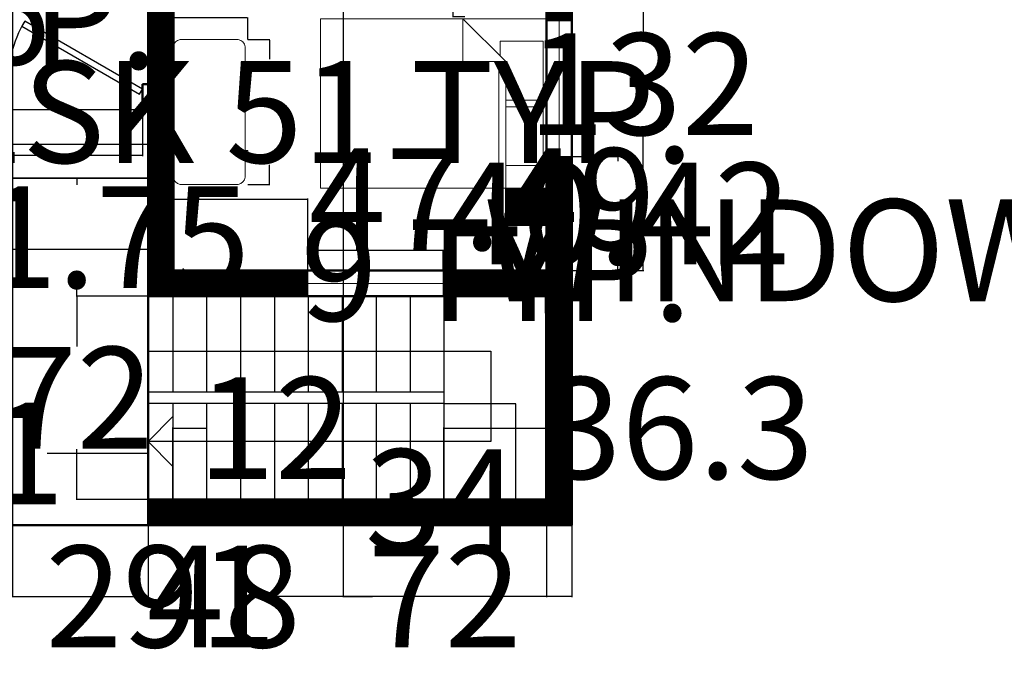
# Model space of a CAD drawing. Units: inches. Extents: x 1173 to 2157, y 515 to 1129.
# Tile 4 of 13: x 1475 to 1824, y 515 to 743. Entities that reach past the tile are written whole.
import ezdxf

# ---------------------------------------------------------------- set-up
doc = ezdxf.new("R2010")
doc.units = ezdxf.units.IN
doc.header["$MEASUREMENT"] = 0
for name, color, linetype, lineweight in [('A-ANNO-DIMS', 2, 'Continuous', 18), ('A-DOOR', 3, 'Continuous', 25), ('A-FLOR', 7, 'Continuous', 25), ('A-FLOR-STRS', 7, 'Continuous', 25), ('A-FURN', 8, 'Continuous', 18), ('A-GLAZ', 4, 'Continuous', 18), ('A-WALL', 7, 'Continuous', 50)]:
    doc.layers.add(name, color=color, linetype=linetype, lineweight=lineweight)
doc.layers.add('A-FURN-PATT', color=7, linetype='Continuous', lineweight=13, true_color=0xffffff)
doc.layers.add('A-WALL-PATT', color=22, linetype='Continuous', lineweight=13, true_color=0xca4b0c)
doc.styles.get("Standard").update_dxf_attribs({"font": 'arial.ttf'})
doc.dimstyles.get("Standard").update_dxf_attribs({"dimtxt": 36, "dimasz": 0.18, "dimexe": 0.18, "dimexo": 0.0625, "dimgap": 0.09, "dimtad": 0, "dimtih": 1, "dimtoh": 1, "dimdec": 0, "dimrnd": 72, "dimzin": 0, "dimdsep": 46, "dimlunit": 3, "dimtxsty": 'Standard', "dimcen": 2, "dimadec": 0, "dimazin": 0, "dimtfac": 1, "dimtdec": 0, "dimtofl": 0, "dimtmove": 0, "dimatfit": 3, "dimfxl": 1, "dimtolj": 1, "dimtzin": 0, "dimarcsym": 0})

# ---------------------------------------------------------------- blocks, each defined once
blk = doc.blocks.new('*U2')
for p, q in [((0, 0), (0, -6)), ((-40, 0), (-40, -6))]:
    blk.add_line(p, q)
blk.add_lwpolyline([(0, 0), (-34.64, 20), (-35.52, 18.48), (-0.88, -1.52)], close=True)
blk.add_arc((0, 0), 40, 150, 180)
blk = doc.blocks.new('Bed - Queen')
for p, q in [((0, -80.00003), (0, 0)), ((0, 0), (59.99999, 0)), ((59.99999, 0), (59.99999, -80.00003)), ((7.99999, -1.2), (28.79998, -1.2)), ((7.99999, -14.4), (7.99999, -1.2)), ((28.79998, -1.2), (28.79998, -14.4)), ((31.19999, -1.2), (51.99999, -1.2)), ((31.19999, -14.4), (31.19999, -1.2)), ((51.99999, -1.2), (51.99999, -16.4)), ((0, -14.4), (44.8, -14.4)), ((44.8, -16.8), (0, -16.8)), ((59.99999, -29.6), (44.8, -14.4)), ((44.8, -14.4), (44.8, -29.6)), ((51.99999, -16.4), (46.79936, -16.4)), ((44.8, -29.6), (59.99999, -29.6)), ((59.99999, -80.00003), (0, -80.00003))]:
    blk.add_line(p, q)
blk = doc.blocks.new('Desk - 30 x 60 in.')
for p, q in [((-26.999995, 0), (26.999995, 0)), ((-29.999995, -27), (-29.999995, -3)), ((29.999995, -3), (29.999995, -27)), ((26.999995, -30), (-26.999995, -30)), ((-20.000005, -30), (-20.000005, -31)), ((-20.000005, -31), (-16.000005, -31)), ((-16.000005, -31), (-16.000005, -30)), ((15.999995, -31), (15.999995, -30)), ((19.999995, -31), (15.999995, -31)), ((19.999995, -30), (19.999995, -31))]:
    blk.add_line(p, q)
for centre, start, end in [((-26.499995, -3.5), 98.1301, 171.8699), ((26.499995, -3.5), 8.130102, 81.8699), ((-26.499995, -26.5), 188.1301, 261.8699), ((26.499995, -26.5), 278.1301, 351.8699)]:
    blk.add_arc(centre, 3.535534, start, end)
blk = doc.blocks.new('WIN-48X9')
blk.add_line((48, 4.5), (0, 4.5))
blk.add_lwpolyline([(0, 9), (48, 9), (48, 0), (0, 0)], close=True)
blk = doc.blocks.new('*D26')
at = {"layer": 'A-ANNO-DIMS', "color": 0, "lineweight": -2, "transparency": 16777216}
for p, q in [((1577.15, 654.34), (1577.15, 661.66)), ((1577.33, 661.48), (1624.97, 661.48)), ((1625.15, 654.34), (1625.15, 661.66)), ((1625.15, 661.48), (1625.33, 661.48))]:
    blk.add_line(p, q, dxfattribs=at)
at = {"layer": 'A-ANNO-DIMS', "color": 0, "transparency": 16777216}
for points in [[(1577.33, 661.51), (1577.33, 661.45), (1577.15, 661.48)], [(1624.97, 661.51), (1624.97, 661.45), (1625.15, 661.48)]]:
    blk.add_solid(points, dxfattribs=at)
at = {"layer": 'Defpoints', "color": 0, "transparency": 16777216}
for p in [(1625.15, 661.48), (1577.15, 654.28), (1625.15, 654.28)]:
    blk.add_point(p, dxfattribs=at)
at = {"layer": 'A-ANNO-DIMS', "color": 0, "transparency": 16777216, "insert": (1831.09, 661.48), "char_height": 36, "attachment_point": 5}
blk.add_mtext('\\A1;WINDOW 48 TYP.', dxfattribs=at)
blk = doc.blocks.new('*D27')
at = {"layer": 'A-ANNO-DIMS', "color": 0, "lineweight": -2, "transparency": 16777216}
for p, q in [((1577.09, 654.28), (1569.77, 654.28)), ((1569.95, 654.28), (1569.95, 654.46)), ((1569.95, 654.46), (1570.13, 654.46)), ((1569.95, 645.46), (1569.95, 654.1)), ((1577.09, 645.28), (1569.77, 645.28))]:
    blk.add_line(p, q, dxfattribs=at)
at = {"layer": 'A-ANNO-DIMS', "color": 0, "transparency": 16777216}
for points in [[(1569.92, 654.1), (1569.98, 654.1), (1569.95, 654.28)], [(1569.92, 645.46), (1569.98, 645.46), (1569.95, 645.28)]]:
    blk.add_solid(points, dxfattribs=at)
at = {"layer": 'Defpoints', "color": 0, "transparency": 16777216}
for p in [(1569.95, 654.28), (1577.15, 654.28), (1577.15, 645.28)]:
    blk.add_point(p, dxfattribs=at)
at = {"layer": 'A-ANNO-DIMS', "color": 0, "transparency": 16777216, "insert": (1643.85, 654.46), "char_height": 36, "attachment_point": 5}
blk.add_mtext('\\A1;9 TYP.', dxfattribs=at)
blk = doc.blocks.new('*D30')
at = {"layer": 'A-ANNO-DIMS', "color": 0, "lineweight": -2, "transparency": 16777216}
for p, q in [((1555.97, 736.03), (1563.78, 736.03)), ((1563.6, 735.85), (1563.6, 729.12)), ((1563.6, 684.97), (1563.6, 691.71)), ((1555.97, 684.79), (1563.78, 684.79))]:
    blk.add_line(p, q, dxfattribs=at)
at = {"layer": 'A-ANNO-DIMS', "color": 0, "transparency": 16777216}
for points in [[(1563.57, 735.85), (1563.63, 735.85), (1563.6, 736.03)], [(1563.57, 684.97), (1563.63, 684.97), (1563.6, 684.79)]]:
    blk.add_solid(points, dxfattribs=at)
at = {"layer": 'Defpoints', "color": 0, "transparency": 16777216}
for p in [(1555.91, 736.03), (1563.6, 736.03), (1555.91, 684.79)]:
    blk.add_point(p, dxfattribs=at)
at = {"layer": 'A-ANNO-DIMS', "color": 0, "transparency": 16777216, "insert": (1563.6, 710.41), "char_height": 36, "attachment_point": 5}
blk.add_mtext('\\A1;DESK 51 TYP.', dxfattribs=at)
blk = doc.blocks.new('*D31')
at = {"layer": 'A-ANNO-DIMS', "color": 0, "lineweight": -2, "transparency": 16777216}
for p, q in [((1529.44, 743.72), (1529.26, 743.72)), ((1529.44, 736.09), (1529.44, 743.9)), ((1555.73, 743.72), (1529.62, 743.72)), ((1555.91, 736.09), (1555.91, 743.9))]:
    blk.add_line(p, q, dxfattribs=at)
at = {"layer": 'A-ANNO-DIMS', "color": 0, "transparency": 16777216}
for points in [[(1529.62, 743.75), (1529.62, 743.69), (1529.44, 743.72)], [(1555.73, 743.75), (1555.73, 743.69), (1555.91, 743.72)]]:
    blk.add_solid(points, dxfattribs=at)
at = {"layer": 'Defpoints', "color": 0, "transparency": 16777216}
for p in [(1529.44, 743.72), (1529.44, 736.03), (1555.91, 736.03)]:
    blk.add_point(p, dxfattribs=at)
at = {"layer": 'A-ANNO-DIMS', "color": 0, "transparency": 16777216, "insert": (1441.24, 743.72), "char_height": 36, "attachment_point": 5}
blk.add_mtext('\\A1;26 TYP.', dxfattribs=at)
blk = doc.blocks.new('*D32')
at = {"layer": 'A-ANNO-DIMS', "color": 0, "lineweight": -2, "transparency": 16777216}
for p, q in [((1632.82, 772.28), (1632.82, 776.62)), ((1633, 776.44), (1660.73, 776.44)), ((1660.91, 772.28), (1660.91, 776.62)), ((1660.91, 776.44), (1661.09, 776.44))]:
    blk.add_line(p, q, dxfattribs=at)
at = {"layer": 'A-ANNO-DIMS', "color": 0, "transparency": 16777216}
for points in [[(1633, 776.47), (1633, 776.41), (1632.82, 776.44)], [(1660.73, 776.47), (1660.73, 776.41), (1660.91, 776.44)]]:
    blk.add_solid(points, dxfattribs=at)
at = {"layer": 'Defpoints', "color": 0, "transparency": 16777216}
for p in [(1660.91, 776.44), (1632.82, 772.22), (1660.91, 772.22)]:
    blk.add_point(p, dxfattribs=at)
at = {"layer": 'A-ANNO-DIMS', "color": 0, "transparency": 16777216, "insert": (1823.46, 776.44), "char_height": 36, "attachment_point": 5}
blk.add_mtext('\\A1;LAMP 28 TYP.', dxfattribs=at)
blk = doc.blocks.new('*D33')
at = {"layer": 'A-ANNO-DIMS', "color": 0, "lineweight": -2, "transparency": 16777216}
for p, q in [((1632.75, 772.22), (1628.42, 772.22)), ((1628.6, 772.22), (1628.6, 772.4)), ((1628.6, 772.4), (1628.78, 772.4)), ((1628.6, 744.31), (1628.6, 772.04)), ((1632.75, 744.13), (1628.42, 744.13))]:
    blk.add_line(p, q, dxfattribs=at)
at = {"layer": 'A-ANNO-DIMS', "color": 0, "transparency": 16777216}
for points in [[(1628.57, 772.04), (1628.63, 772.04), (1628.6, 772.22)], [(1628.57, 744.31), (1628.63, 744.31), (1628.6, 744.13)]]:
    blk.add_solid(points, dxfattribs=at)
at = {"layer": 'Defpoints', "color": 0, "transparency": 16777216}
for p in [(1628.6, 772.22), (1632.82, 772.22), (1632.82, 744.13)]:
    blk.add_point(p, dxfattribs=at)
at = {"layer": 'A-ANNO-DIMS', "color": 0, "transparency": 16777216, "insert": (1716.8, 772.4), "char_height": 36, "attachment_point": 5}
blk.add_mtext('\\A1;28 TYP.', dxfattribs=at)
blk = doc.blocks.new('*D50')
at = {"layer": 'A-ANNO-DIMS', "color": 0, "lineweight": -2, "transparency": 16777216}
for p, q in [((1603.33, 796.77), (1603.15, 796.77)), ((1603.33, 798.21), (1603.33, 796.59)), ((1613.15, 796.77), (1603.51, 796.77)), ((1613.33, 798.21), (1613.33, 796.59))]:
    blk.add_line(p, q, dxfattribs=at)
at = {"layer": 'A-ANNO-DIMS', "color": 0, "transparency": 16777216}
for points in [[(1603.51, 796.8), (1603.51, 796.74), (1603.33, 796.77)], [(1613.15, 796.8), (1613.15, 796.74), (1613.33, 796.77)]]:
    blk.add_solid(points, dxfattribs=at)
at = {"layer": 'Defpoints', "color": 0, "transparency": 16777216}
for p in [(1603.33, 798.27), (1603.33, 796.77), (1613.33, 798.27)]:
    blk.add_point(p, dxfattribs=at)
at = {"layer": 'A-ANNO-DIMS', "color": 0, "transparency": 16777216, "insert": (1377.9, 796.77), "char_height": 36, "attachment_point": 5}
blk.add_mtext('\\A1;BASIN TAP 10 TYP.', dxfattribs=at)
blk = doc.blocks.new('*D64')
at = {"layer": 'A-ANNO-DIMS', "color": 0, "lineweight": -2, "transparency": 16777216}
for p, q in [((1379.66, 564.22), (1379.66, 538.8)), ((1670.66, 564.22), (1670.66, 538.8)), ((1379.84, 538.98), (1488.47, 538.98)), ((1670.48, 538.98), (1561.86, 538.98))]:
    blk.add_line(p, q, dxfattribs=at)
at = {"layer": 'A-ANNO-DIMS', "color": 0, "transparency": 16777216}
for points in [[(1379.84, 539.01), (1379.84, 538.95), (1379.66, 538.98)], [(1670.48, 539.01), (1670.48, 538.95), (1670.66, 538.98)]]:
    blk.add_solid(points, dxfattribs=at)
at = {"layer": 'Defpoints', "color": 0, "transparency": 16777216}
for p in [(1379.66, 564.28), (1670.66, 564.28), (1670.66, 538.98)]:
    blk.add_point(p, dxfattribs=at)
at = {"layer": 'A-ANNO-DIMS', "color": 0, "transparency": 16777216, "insert": (1525.16, 538.98), "char_height": 36, "attachment_point": 5}
blk.add_mtext('\\A1;291', dxfattribs=at)
blk = doc.blocks.new('*D69')
at = {"layer": 'A-ANNO-DIMS', "color": 0, "lineweight": -2, "transparency": 16777216}
for p, q in [((1472.66, 924.22), (1472.66, 538.8)), ((1520.66, 924.22), (1520.66, 538.8)), ((1472.84, 538.98), (1520.48, 538.98)), ((1520.66, 538.98), (1520.84, 538.98))]:
    blk.add_line(p, q, dxfattribs=at)
at = {"layer": 'A-ANNO-DIMS', "color": 0, "transparency": 16777216}
for points in [[(1472.84, 539.01), (1472.84, 538.95), (1472.66, 538.98)], [(1520.48, 539.01), (1520.48, 538.95), (1520.66, 538.98)]]:
    blk.add_solid(points, dxfattribs=at)
at = {"layer": 'Defpoints', "color": 0, "transparency": 16777216}
for p in [(1472.66, 924.28), (1520.66, 924.28), (1520.66, 538.98)]:
    blk.add_point(p, dxfattribs=at)
at = {"layer": 'A-ANNO-DIMS', "color": 0, "transparency": 16777216, "insert": (1547.48, 538.98), "char_height": 36, "attachment_point": 5}
blk.add_mtext('\\A1;48', dxfattribs=at)
blk = doc.blocks.new('*D71')
at = {"layer": 'A-ANNO-DIMS', "color": 0, "lineweight": -2, "transparency": 16777216}
for p, q in [((1453.65, 686.97), (1453.65, 661.55)), ((1520.66, 686.97), (1520.66, 661.55)), ((1453.65, 661.73), (1453.47, 661.73)), ((1520.48, 661.73), (1453.83, 661.73))]:
    blk.add_line(p, q, dxfattribs=at)
at = {"layer": 'A-ANNO-DIMS', "color": 0, "transparency": 16777216}
for points in [[(1453.83, 661.76), (1453.83, 661.7), (1453.65, 661.73)], [(1520.48, 661.76), (1520.48, 661.7), (1520.66, 661.73)]]:
    blk.add_solid(points, dxfattribs=at)
at = {"layer": 'Defpoints', "color": 0, "transparency": 16777216}
for p in [(1453.65, 687.03), (1520.66, 687.03), (1453.65, 661.73)]:
    blk.add_point(p, dxfattribs=at)
at = {"layer": 'A-ANNO-DIMS', "color": 0, "transparency": 16777216, "insert": (1396.02, 661.73), "char_height": 36, "attachment_point": 5}
blk.add_mtext('\\A1;67.01', dxfattribs=at)
blk = doc.blocks.new('*D72')
at = {"layer": 'A-ANNO-DIMS', "color": 0, "lineweight": -2, "transparency": 16777216}
for p, q in [((1470.66, 720.22), (1470.66, 694.8)), ((1518.66, 720.22), (1518.66, 694.8)), ((1470.66, 694.98), (1470.48, 694.98)), ((1518.48, 694.98), (1470.84, 694.98))]:
    blk.add_line(p, q, dxfattribs=at)
at = {"layer": 'A-ANNO-DIMS', "color": 0, "transparency": 16777216}
for points in [[(1470.84, 695.01), (1470.84, 694.95), (1470.66, 694.98)], [(1518.48, 695.01), (1518.48, 694.95), (1518.66, 694.98)]]:
    blk.add_solid(points, dxfattribs=at)
at = {"layer": 'Defpoints', "color": 0, "transparency": 16777216}
for p in [(1470.66, 720.28), (1518.66, 720.28), (1470.66, 694.98)]:
    blk.add_point(p, dxfattribs=at)
at = {"layer": 'A-ANNO-DIMS', "color": 0, "transparency": 16777216, "insert": (1443.85, 694.98), "char_height": 36, "attachment_point": 5}
blk.add_mtext('\\A1;48', dxfattribs=at)
blk = doc.blocks.new('*D73')
at = {"layer": 'A-ANNO-DIMS', "color": 0, "lineweight": -2, "transparency": 16777216}
for p, q in [((1379.66, 564.34), (1379.66, 589.76)), ((1379.84, 589.58), (1415.47, 589.58)), ((1520.48, 589.58), (1484.85, 589.58)), ((1520.66, 564.34), (1520.66, 589.76))]:
    blk.add_line(p, q, dxfattribs=at)
at = {"layer": 'A-ANNO-DIMS', "color": 0, "transparency": 16777216}
for points in [[(1379.84, 589.61), (1379.84, 589.55), (1379.66, 589.58)], [(1520.48, 589.61), (1520.48, 589.55), (1520.66, 589.58)]]:
    blk.add_solid(points, dxfattribs=at)
at = {"layer": 'Defpoints', "color": 0, "transparency": 16777216}
for p in [(1520.66, 589.58), (1379.66, 564.28), (1520.66, 564.28)]:
    blk.add_point(p, dxfattribs=at)
at = {"layer": 'A-ANNO-DIMS', "color": 0, "transparency": 16777216, "insert": (1450.16, 589.58), "char_height": 36, "attachment_point": 5}
blk.add_mtext('\\A1;141', dxfattribs=at)
blk = doc.blocks.new('*D74')
at = {"layer": 'A-ANNO-DIMS', "color": 0, "lineweight": -2, "transparency": 16777216}
for p, q in [((1529.37, 573.34), (1529.37, 598.76)), ((1529.55, 598.58), (1541.19, 598.58)), ((1541.37, 573.34), (1541.37, 598.76)), ((1541.37, 598.58), (1541.55, 598.58))]:
    blk.add_line(p, q, dxfattribs=at)
at = {"layer": 'A-ANNO-DIMS', "color": 0, "transparency": 16777216}
for points in [[(1529.55, 598.61), (1529.55, 598.55), (1529.37, 598.58)], [(1541.19, 598.61), (1541.19, 598.55), (1541.37, 598.58)]]:
    blk.add_solid(points, dxfattribs=at)
at = {"layer": 'Defpoints', "color": 0, "transparency": 16777216}
for p in [(1541.37, 598.58), (1529.37, 573.28), (1541.37, 573.28)]:
    blk.add_point(p, dxfattribs=at)
at = {"layer": 'A-ANNO-DIMS', "color": 0, "transparency": 16777216, "insert": (1565.54, 598.58), "char_height": 36, "attachment_point": 5}
blk.add_mtext('\\A1;12', dxfattribs=at)
blk = doc.blocks.new('*D75')
at = {"layer": 'A-ANNO-DIMS', "color": 0, "lineweight": -2, "transparency": 16777216}
for p, q in [((1625.37, 573.34), (1625.37, 598.76)), ((1625.55, 598.58), (1661.48, 598.58)), ((1661.66, 573.34), (1661.66, 598.76)), ((1661.66, 598.58), (1661.84, 598.58))]:
    blk.add_line(p, q, dxfattribs=at)
at = {"layer": 'A-ANNO-DIMS', "color": 0, "transparency": 16777216}
for points in [[(1625.55, 598.61), (1625.55, 598.55), (1625.37, 598.58)], [(1661.48, 598.61), (1661.48, 598.55), (1661.66, 598.58)]]:
    blk.add_solid(points, dxfattribs=at)
at = {"layer": 'Defpoints', "color": 0, "transparency": 16777216}
for p in [(1661.66, 598.58), (1625.37, 573.28), (1661.66, 573.28)]:
    blk.add_point(p, dxfattribs=at)
at = {"layer": 'A-ANNO-DIMS', "color": 0, "transparency": 16777216, "insert": (1708.68, 598.58), "char_height": 36, "attachment_point": 5}
blk.add_mtext('\\A1;36.3', dxfattribs=at)
blk = doc.blocks.new('*D76')
at = {"layer": 'A-ANNO-DIMS', "color": 0, "lineweight": -2, "transparency": 16777216}
for p, q in [((1625.43, 607.28), (1650.85, 607.28)), ((1650.67, 607.1), (1650.67, 573.46)), ((1625.43, 573.28), (1650.85, 573.28)), ((1650.67, 573.1), (1650.49, 573.1)), ((1650.67, 573.28), (1650.67, 573.1))]:
    blk.add_line(p, q, dxfattribs=at)
at = {"layer": 'A-ANNO-DIMS', "color": 0, "transparency": 16777216}
for points in [[(1650.64, 607.1), (1650.7, 607.1), (1650.67, 607.28)], [(1650.64, 573.46), (1650.7, 573.46), (1650.67, 573.28)]]:
    blk.add_solid(points, dxfattribs=at)
at = {"layer": 'Defpoints', "color": 0, "transparency": 16777216}
for p in [(1625.37, 607.28), (1625.37, 573.28), (1650.67, 573.28)]:
    blk.add_point(p, dxfattribs=at)
at = {"layer": 'A-ANNO-DIMS', "color": 0, "transparency": 16777216, "insert": (1624.7, 573.1), "char_height": 36, "attachment_point": 5}
blk.add_mtext('\\A1;34', dxfattribs=at)
blk = doc.blocks.new('*D77')
at = {"layer": 'A-ANNO-DIMS', "color": 0, "lineweight": -2, "transparency": 16777216}
for p, q in [((1520.6, 645.28), (1495.18, 645.28)), ((1495.36, 645.1), (1495.36, 627.44)), ((1495.36, 573.46), (1495.36, 591.12)), ((1520.6, 573.28), (1495.18, 573.28))]:
    blk.add_line(p, q, dxfattribs=at)
at = {"layer": 'A-ANNO-DIMS', "color": 0, "transparency": 16777216}
for points in [[(1495.33, 645.1), (1495.39, 645.1), (1495.36, 645.28)], [(1495.33, 573.46), (1495.39, 573.46), (1495.36, 573.28)]]:
    blk.add_solid(points, dxfattribs=at)
at = {"layer": 'Defpoints', "color": 0, "transparency": 16777216}
for p in [(1495.36, 645.28), (1520.66, 645.28), (1520.66, 573.28)]:
    blk.add_point(p, dxfattribs=at)
at = {"layer": 'A-ANNO-DIMS', "color": 0, "transparency": 16777216, "insert": (1495.36, 609.28), "char_height": 36, "attachment_point": 5}
blk.add_mtext('\\A1;72', dxfattribs=at)
blk = doc.blocks.new('*D78')
at = {"layer": 'A-ANNO-DIMS', "color": 0, "lineweight": -2, "transparency": 16777216}
for p, q in [((1520.6, 687.03), (1495.18, 687.03)), ((1495.36, 686.85), (1495.36, 684.63)), ((1520.6, 645.28), (1495.18, 645.28)), ((1495.36, 645.46), (1495.36, 647.69))]:
    blk.add_line(p, q, dxfattribs=at)
at = {"layer": 'A-ANNO-DIMS', "color": 0, "transparency": 16777216}
for points in [[(1495.33, 686.85), (1495.39, 686.85), (1495.36, 687.03)], [(1495.33, 645.46), (1495.39, 645.46), (1495.36, 645.28)]]:
    blk.add_solid(points, dxfattribs=at)
at = {"layer": 'Defpoints', "color": 0, "transparency": 16777216}
for p in [(1495.36, 687.03), (1520.66, 687.03), (1520.66, 645.28)]:
    blk.add_point(p, dxfattribs=at)
at = {"layer": 'A-ANNO-DIMS', "color": 0, "transparency": 16777216, "insert": (1495.36, 666.16), "char_height": 36, "attachment_point": 5}
blk.add_mtext('\\A1;41.75', dxfattribs=at)
blk = doc.blocks.new('*D80')
at = {"layer": 'A-ANNO-DIMS', "color": 0, "lineweight": -2, "transparency": 16777216}
for p, q in [((1388.6, 745.04), (1363.18, 745.04)), ((1363.36, 745.04), (1363.36, 745.22)), ((1363.36, 745.22), (1363.54, 745.22)), ((1363.36, 720.46), (1363.36, 744.86)), ((1388.6, 720.28), (1363.18, 720.28))]:
    blk.add_line(p, q, dxfattribs=at)
at = {"layer": 'A-ANNO-DIMS', "color": 0, "transparency": 16777216}
for points in [[(1363.33, 744.86), (1363.39, 744.86), (1363.36, 745.04)], [(1363.33, 720.46), (1363.39, 720.46), (1363.36, 720.28)]]:
    blk.add_solid(points, dxfattribs=at)
at = {"layer": 'Defpoints', "color": 0, "transparency": 16777216}
for p in [(1363.36, 745.04), (1388.66, 745.04), (1388.66, 720.28)]:
    blk.add_point(p, dxfattribs=at)
at = {"layer": 'A-ANNO-DIMS', "color": 0, "transparency": 16777216, "insert": (1424.67, 745.22), "char_height": 36, "attachment_point": 5}
blk.add_mtext('\\A1;24.76', dxfattribs=at)
blk = doc.blocks.new('*D83')
at = {"layer": 'A-ANNO-DIMS', "color": 0, "lineweight": -2, "transparency": 16777216}
for p, q in [((1661.73, 694.7), (1687.15, 694.7)), ((1686.97, 694.52), (1686.97, 692.96)), ((1686.97, 654.46), (1686.97, 656.02)), ((1661.73, 654.28), (1687.15, 654.28))]:
    blk.add_line(p, q, dxfattribs=at)
at = {"layer": 'A-ANNO-DIMS', "color": 0, "transparency": 16777216}
for points in [[(1686.94, 694.52), (1687, 694.52), (1686.97, 694.7)], [(1686.94, 654.46), (1687, 654.46), (1686.97, 654.28)]]:
    blk.add_solid(points, dxfattribs=at)
at = {"layer": 'Defpoints', "color": 0, "transparency": 16777216}
for p in [(1661.66, 694.7), (1661.66, 654.28), (1686.97, 654.28)]:
    blk.add_point(p, dxfattribs=at)
at = {"layer": 'A-ANNO-DIMS', "color": 0, "transparency": 16777216, "insert": (1686.97, 674.49), "char_height": 36, "attachment_point": 5}
blk.add_mtext('\\A1;40.42', dxfattribs=at)
blk = doc.blocks.new('*D84')
at = {"layer": 'A-ANNO-DIMS', "color": 0, "lineweight": -2, "transparency": 16777216}
for p, q in [((1661.73, 786.28), (1696.15, 786.28)), ((1695.97, 786.1), (1695.97, 738.76)), ((1695.97, 654.46), (1695.97, 701.8)), ((1661.73, 654.28), (1696.15, 654.28))]:
    blk.add_line(p, q, dxfattribs=at)
at = {"layer": 'A-ANNO-DIMS', "color": 0, "transparency": 16777216}
for points in [[(1695.94, 786.1), (1696, 786.1), (1695.97, 786.28)], [(1695.94, 654.46), (1696, 654.46), (1695.97, 654.28)]]:
    blk.add_solid(points, dxfattribs=at)
at = {"layer": 'Defpoints', "color": 0, "transparency": 16777216}
for p in [(1661.66, 786.28), (1661.66, 654.28), (1695.97, 654.28)]:
    blk.add_point(p, dxfattribs=at)
at = {"layer": 'A-ANNO-DIMS', "color": 0, "transparency": 16777216, "insert": (1695.97, 720.28), "char_height": 36, "attachment_point": 5}
blk.add_mtext('\\A1;132', dxfattribs=at)
blk = doc.blocks.new('*D85')
at = {"layer": 'A-ANNO-DIMS', "color": 0, "lineweight": -2, "transparency": 16777216}
for p, q in [((1529.66, 654.34), (1529.66, 679.76)), ((1529.84, 679.58), (1576.97, 679.58)), ((1577.15, 654.34), (1577.15, 679.76)), ((1577.15, 679.58), (1577.33, 679.58))]:
    blk.add_line(p, q, dxfattribs=at)
at = {"layer": 'A-ANNO-DIMS', "color": 0, "transparency": 16777216}
for points in [[(1529.84, 679.61), (1529.84, 679.55), (1529.66, 679.58)], [(1576.97, 679.61), (1576.97, 679.55), (1577.15, 679.58)]]:
    blk.add_solid(points, dxfattribs=at)
at = {"layer": 'Defpoints', "color": 0, "transparency": 16777216}
for p in [(1577.15, 679.58), (1529.66, 654.28), (1577.15, 654.28)]:
    blk.add_point(p, dxfattribs=at)
at = {"layer": 'A-ANNO-DIMS', "color": 0, "transparency": 16777216, "insert": (1638.92, 679.58), "char_height": 36, "attachment_point": 5}
blk.add_mtext('\\A1;47.49', dxfattribs=at)
blk = doc.blocks.new('*D95')
at = {"layer": 'A-ANNO-DIMS', "color": 0, "lineweight": -2, "transparency": 16777216}
for p, q in [((1589.66, 795.22), (1589.66, 538.8)), ((1661.66, 795.22), (1661.66, 538.8)), ((1589.84, 538.98), (1600.12, 538.98)), ((1661.48, 538.98), (1651.21, 538.98))]:
    blk.add_line(p, q, dxfattribs=at)
at = {"layer": 'A-ANNO-DIMS', "color": 0, "transparency": 16777216}
for points in [[(1589.84, 539.01), (1589.84, 538.95), (1589.66, 538.98)], [(1661.48, 539.01), (1661.48, 538.95), (1661.66, 538.98)]]:
    blk.add_solid(points, dxfattribs=at)
at = {"layer": 'Defpoints', "color": 0, "transparency": 16777216}
for p in [(1589.66, 795.28), (1661.66, 795.28), (1661.66, 538.98)]:
    blk.add_point(p, dxfattribs=at)
at = {"layer": 'A-ANNO-DIMS', "color": 0, "transparency": 16777216, "insert": (1625.66, 538.98), "char_height": 36, "attachment_point": 5}
blk.add_mtext('\\A1;72', dxfattribs=at)

msp = doc.modelspace()

# ---------------------------------------------------------------- hatches: boundary and pattern name
at = {"layer": 'A-FURN-PATT'}
h = msp.add_hatch(dxfattribs=at)
h.set_pattern_fill('ANSI31', color=256)
h.paths.add_polyline_path([(1661.6635, 683.432), (1647.1943, 683.432), (1647.1943, 670.2263), (1661.6635, 670.2263)])
at = {"layer": 'A-WALL-PATT'}
h = msp.add_hatch(dxfattribs=at)
h.set_pattern_fill('ANSI31', color=256)
h.paths.add_polyline_path([(1388.6635, 933.2805), (1388.6635, 1044.2805), (1413.7618, 1044.2805), (1413.7618, 1053.2805), (1379.6635, 1053.2805), (1379.6635, 894.1606), (1388.6635, 894.1606), (1388.6635, 924.2805), (1472.6635, 924.2805), (1472.6635, 933.2805)])
h.paths.add_polyline_path([(1520.6635, 1044.2805), (1520.6635, 1014.7866), (1520.6635, 1005.1794), (1520.7714, 1005.1794), (1520.7714, 956.4707), (1520.6635, 924.2805), (1529.6635, 924.2805), (1529.6635, 931.4788), (1529.6635, 1044.2805), (1530.8474, 1044.2805), (1570.9543, 1044.2805), (1570.9543, 1053.2805), (1461.7618, 1053.2805), (1461.7618, 1044.2805)])
h.paths.add_polyline_path([(1618.9543, 1053.2805), (1618.9543, 1044.2805), (1661.6635, 1044.2805), (1661.6635, 1043.7367), (1661.6635, 1032.8874), (1670.6635, 1032.8874), (1670.6635, 1053.2805)])
h.paths.add_polyline_path([(1661.6635, 933.2805), (1661.6635, 927.8377), (1661.6635, 924.2805), (1661.6635, 918.9156), (1670.6635, 918.9156), (1670.6635, 984.8874), (1661.6635, 984.8874), (1661.6635, 978.3712)])
h.paths.add_polyline_path([(1670.6635, 894.9156), (1661.6635, 894.9156), (1661.6635, 890.0349), (1661.9328, 890.0349), (1661.9328, 870.079), (1661.6635, 864.2805), (1589.6635, 864.2805), (1589.6635, 924.2805), (1625.553, 924.2805, -0.02455299), (1625.3782, 927.8377), (1625.3782, 933.2805), (1577.6635, 933.2805), (1577.6635, 924.2805), (1580.6635, 924.2805), (1580.6635, 855.2805), (1586.1062, 855.2805), (1589.6635, 855.2805), (1661.6635, 855.2805), (1661.6635, 826.5597), (1670.6635, 826.5597)])
h.paths.add_polyline_path([(1670.6635, 802.5597), (1661.6635, 802.5597), (1661.6635, 795.2805), (1589.6635, 795.2805), (1589.6635, 819.17, -0.02455299), (1586.1062, 818.9952), (1580.6635, 818.9952), (1580.6635, 795.2805), (1577.6635, 795.2805), (1577.6635, 786.2805), (1661.6635, 786.2805), (1661.6635, 778.5597), (1661.6635, 742.6973), (1670.6635, 742.6973)])
h.paths.add_polyline_path([(1661.6635, 654.2805), (1625.1498, 654.2805), (1625.1498, 645.2805), (1661.3656, 645.2805), (1661.6635, 645.2805), (1661.6635, 573.2805), (1520.6635, 573.2805), (1520.6635, 564.2805), (1670.6635, 564.2805), (1670.6635, 694.6973), (1661.6635, 694.6973)])
h.paths.add_polyline_path([(1529.4367, 733.4702, -0.06854064), (1529.6635, 734.2623), (1529.6635, 795.2805), (1520.6635, 795.2805), (1520.6635, 645.2805), (1577.1498, 645.2805), (1577.1498, 654.2805), (1529.6635, 654.2805), (1529.6635, 686.5626, -0.06854064), (1529.4367, 687.3547)])
h.paths.add_polyline_path([(1379.6635, 711.2805), (1388.6635, 711.2805), (1458.7214, 711.2805), (1458.7214, 720.2805), (1410.7214, 720.2805), (1388.6635, 720.2805), (1388.6635, 745.0427), (1379.6635, 745.0427)])
h.paths.add_polyline_path([(1388.6635, 846.1606), (1379.6635, 846.1606), (1379.6635, 793.0427), (1388.6635, 793.0427)])

# ---------------------------------------------------------------- linework, layer by layer
at = {"layer": 'A-FLOR'}
for p, q in [((1453.6517, 687.0336), (1520.6635, 687.0336)), ((1520.6635, 687.0336), (1520.6635, 568.7805)), ((1520.6635, 568.7805), (1520.6635, 564.2805)), ((1520.6635, 564.2805), (1379.6635, 564.2805))]:
    msp.add_line(p, q, dxfattribs=at)
at = {"layer": 'A-FLOR-STRS'}
for p, q in [((1470.6635, 711.2805), (1520.6635, 711.2805)), ((1453.6517, 699.0155), (1520.6635, 699.0155)), ((1520.6635, 699.0155), (1520.6635, 687.0336)), ((1520.6635, 687.0336), (1453.6517, 687.0336)), ((1529.3656, 645.2805), (1529.3656, 611.2805)), ((1541.3656, 645.2805), (1529.3656, 645.2805)), ((1661.3656, 645.2805), (1541.3656, 645.2805)), ((1541.3656, 645.2805), (1661.3656, 645.2805)), ((1541.3656, 645.2805), (1541.3656, 611.2805)), ((1553.3656, 645.2805), (1553.3656, 611.2805)), ((1565.3656, 645.2805), (1565.3656, 611.2805)), ((1577.3656, 645.2805), (1577.3656, 611.2805)), ((1589.3656, 645.2805), (1589.3656, 611.2805)), ((1601.3656, 645.2805), (1601.3656, 611.2805)), ((1613.3656, 645.2805), (1613.3656, 611.2805)), ((1625.3656, 645.2805), (1625.3656, 573.2805)), ((1661.3656, 645.2805), (1661.3656, 639.2805)), ((1661.3656, 639.2805), (1661.3656, 645.2805)), ((1661.3656, 645.2805), (1661.3656, 573.2805)), ((1520.6635, 625.7636), (1641.9658, 625.7636)), ((1641.9658, 625.7636), (1641.9658, 593.8272)), ((1589.3656, 611.2805), (1520.6635, 611.2805)), ((1625.3656, 611.2805), (1589.3656, 611.2805)), ((1589.3656, 607.2805), (1520.6635, 607.2805)), ((1529.3656, 607.2805), (1529.3656, 573.2805)), ((1541.3656, 607.2805), (1541.3656, 573.2805)), ((1553.3656, 607.2805), (1553.3656, 573.2805)), ((1565.3656, 607.2805), (1565.3656, 573.2805)), ((1577.3656, 607.2805), (1577.3656, 573.2805)), ((1625.3656, 607.2805), (1589.3656, 607.2805)), ((1589.3656, 607.2805), (1589.3656, 573.2805)), ((1601.3656, 607.2805), (1601.3656, 573.2805)), ((1613.3656, 607.2805), (1613.3656, 573.2805)), ((1529.3675, 602.673), (1520.6653, 593.8253)), ((1641.9658, 593.8272), (1520.6635, 593.8272)), ((1529.3675, 584.9775), (1520.6635, 593.8272)), ((1589.3656, 573.2805), (1529.3656, 573.2805)), ((1661.3656, 573.2805), (1589.3656, 573.2805))]:
    msp.add_line(p, q, dxfattribs=at)
at = {"layer": 'A-FURN'}
msp.add_lwpolyline([(1661.6635, 683.432), (1647.1943, 683.432), (1647.1943, 670.2263), (1661.6635, 670.2263)], close=True, dxfattribs=at)
at = {"layer": 'A-WALL'}
for p, q in [((1520.6635, 645.2805), (1520.6635, 795.2805)), ((1529.6635, 654.2805), (1529.6635, 795.2805)), ((1661.6635, 654.2805), (1661.6635, 786.2805)), ((1520.6635, 720.2805), (1518.6635, 720.2805)), ((1518.6635, 711.2805), (1518.6635, 720.2805)), ((1520.6635, 711.2805), (1518.6635, 711.2805)), ((1661.6635, 654.2805), (1529.6635, 654.2805)), ((1661.6635, 645.2805), (1520.6635, 645.2805)), ((1520.6635, 645.2805), (1520.6635, 573.2805)), ((1661.6635, 573.2805), (1661.6635, 645.2805)), ((1520.6635, 573.2805), (1661.6635, 573.2805)), ((1520.6635, 573.2805), (1520.6635, 564.2805))]:
    msp.add_line(p, q, dxfattribs=at)
msp.add_lwpolyline([(1379.6635, 564.2805), (1670.6635, 564.2805), (1670.6635, 1053.2805), (1379.6635, 1053.2805)], close=True, dxfattribs=at)

# ---------------------------------------------------------------- block references
at = {"layer": 'A-DOOR', "xscale": 1.204044770816111, "yscale": 1.204044770816111, "zscale": 1.204044770816111}
msp.add_blockref('*U2', (1518.6635, 718.5048), dxfattribs=at)
at = {"layer": 'A-FURN', "xscale": -1, "rotation": 270}
msp.add_blockref('Bed - Queen', (1661.6635, 683.432), dxfattribs=at)
at = {"layer": 'A-FURN', "xscale": 0.8539907571596934, "yscale": 0.8539907571596934, "zscale": 0.8539907571596934, "rotation": 90}
msp.add_blockref('Desk - 30 x 60 in.', (1529.4367, 710.4125), dxfattribs=at)
at = {"layer": 'A-GLAZ', "rotation": 270.0000000000009}
msp.add_blockref('WIN-48X9', (1661.6635, 742.6973), dxfattribs=at)
at = {"layer": 'A-GLAZ'}
msp.add_blockref('WIN-48X9', (1577.1498, 645.2805), dxfattribs=at)

# ---------------------------------------------------------------- dimensions: what is measured, and where the dimension line sits
at = {"layer": 'A-ANNO-DIMS'}
for base, p1, p2, override, picture, middle in [((1520.6635, 538.978), (1472.6635, 924.2805), (1520.6635, 924.2805), {"dimdec": 0, "dimlfac": 1, "dimrnd": 0, "dimzin": 0, "dimdsep": 46, "dimlunit": 2}, '*D69', (1547.4792, 538.978)), ((1661.6635, 538.978), (1589.6635, 795.2805), (1661.6635, 795.2805), {"dimdec": 0, "dimlfac": 1, "dimrnd": 0, "dimzin": 0, "dimdsep": 46, "dimlunit": 2}, '*D95', (1625.6635, 538.978)), ((1577.1498, 679.583), (1529.6635, 654.2805), (1577.1498, 654.2805), {"dimdec": 2, "dimlfac": 1, "dimrnd": 0, "dimzin": 0, "dimdsep": 46, "dimlunit": 2}, '*D85', (1638.9219, 679.583)), ((1541.3656, 598.583), (1529.3656, 573.2805), (1541.3656, 573.2805), {"dimdec": 0, "dimlfac": 1, "dimrnd": 0, "dimzin": 0, "dimdsep": 46, "dimlunit": 2}, '*D74', (1565.5415, 598.583)), ((1661.6635, 598.583), (1625.3656, 573.2805), (1661.6635, 573.2805), {"dimdec": 1, "dimlfac": 1, "dimrnd": 0, "dimzin": 0, "dimdsep": 46, "dimlunit": 2}, '*D75', (1708.677, 598.583)), ((1520.6635, 589.583), (1379.6635, 564.2805), (1520.6635, 564.2805), {"dimdec": 0, "dimlfac": 1, "dimrnd": 0, "dimzin": 0, "dimdsep": 46, "dimlunit": 2}, '*D73', (1450.1635, 589.583)), ((1670.6635, 538.978), (1379.6635, 564.2805), (1670.6635, 564.2805), {"dimdec": 0, "dimlfac": 1, "dimrnd": 0, "dimzin": 0, "dimdsep": 46, "dimlunit": 2}, '*D64', (1525.1635, 538.978))]:
    dim = msp.add_linear_dim(base=base, p1=p1, p2=p2, dimstyle='Standard', override=override, dxfattribs=at)
    dim.commit()
    dim.dimension.update_dxf_attribs({"geometry": picture, "text_midpoint": middle})
for base, p1, p2, angle, text, picture, middle in [((1603.3335, 796.7679), (1613.3335, 798.2679), (1603.3335, 798.2679), 180, 'BASIN TAP <> TYP.', '*D50', (1377.9039, 796.7679)), ((1628.6024, 772.2213), (1632.8165, 744.1274), (1632.8165, 772.2213), 90, '<> TYP.', '*D33', (1716.7974, 772.4013)), ((1529.4367, 743.7181), (1555.9105, 736.0322), (1529.4367, 736.0322), 180, '<> TYP.', '*D31', (1441.2418, 743.7181)), ((1563.5964, 736.0322), (1555.9105, 684.7928), (1555.9105, 736.0322), 90, 'DESK <> TYP.', '*D30', (1563.5964, 710.4125)), ((1569.9498, 654.2805), (1577.1498, 645.2805), (1577.1498, 654.2805), 90, '<> TYP.', '*D27', (1643.8529, 654.4605))]:
    dim = msp.add_linear_dim(base=base, p1=p1, p2=p2, angle=angle, text=text, dimstyle='Standard', override={"dimdec": 0, "dimlfac": 1, "dimrnd": 0, "dimzin": 0, "dimdsep": 46, "dimlunit": 2}, dxfattribs=at)
    dim.commit()
    dim.dimension.update_dxf_attribs({"geometry": picture, "text_midpoint": middle})
for base, p1, p2, text, picture, middle in [((1660.9104, 776.4354), (1632.8165, 772.2213), (1660.9104, 772.2213), 'LAMP <> TYP.', '*D32', (1823.4628, 776.4354)), ((1625.1498, 661.4805), (1577.1498, 654.2805), (1625.1498, 654.2805), 'WINDOW <> TYP.', '*D26', (1831.0938, 661.4805))]:
    dim = msp.add_linear_dim(base=base, p1=p1, p2=p2, text=text, dimstyle='Standard', override={"dimdec": 0, "dimlfac": 1, "dimrnd": 0, "dimzin": 0, "dimdsep": 46, "dimlunit": 2}, dxfattribs=at)
    dim.commit()
    dim.dimension.update_dxf_attribs({"geometry": picture, "text_midpoint": middle})
for base, p1, p2, angle, override, picture, middle in [((1695.966, 654.2805), (1661.6635, 786.2805), (1661.6635, 654.2805), 90, {"dimdec": 0, "dimlfac": 1, "dimrnd": 0, "dimzin": 0, "dimdsep": 46, "dimlunit": 2}, '*D84', (1695.966, 720.2805)), ((1363.361, 745.0427), (1388.6635, 720.2805), (1388.6635, 745.0427), 90, {"dimdec": 2, "dimlfac": 1, "dimrnd": 0, "dimzin": 0, "dimdsep": 46, "dimlunit": 2}, '*D80', (1424.6664, 745.2227)), ((1470.6635, 694.978), (1518.6635, 720.2805), (1470.6635, 720.2805), 180, {"dimdec": 0, "dimlfac": 1, "dimrnd": 0, "dimzin": 0, "dimdsep": 46, "dimlunit": 2}, '*D72', (1443.8478, 694.978)), ((1686.966, 654.2805), (1661.6635, 694.6973), (1661.6635, 654.2805), 270, {"dimdec": 2, "dimlfac": 1, "dimrnd": 0, "dimzin": 0, "dimdsep": 46, "dimlunit": 2}, '*D83', (1686.966, 674.4889)), ((1453.6517, 661.7311), (1520.6635, 687.0336), (1453.6517, 687.0336), 180, {"dimdec": 2, "dimlfac": 1, "dimrnd": 0, "dimzin": 0, "dimdsep": 46, "dimlunit": 2}, '*D71', (1396.0175, 661.7311)), ((1495.361, 687.0336), (1520.6635, 645.2805), (1520.6635, 687.0336), 90, {"dimdec": 2, "dimlfac": 1, "dimrnd": 0, "dimzin": 0, "dimdsep": 46, "dimlunit": 2}, '*D78', (1495.361, 666.1571)), ((1495.361, 645.2805), (1520.6635, 573.2805), (1520.6635, 645.2805), 90, {"dimdec": 0, "dimlfac": 1, "dimrnd": 0, "dimzin": 0, "dimdsep": 46, "dimlunit": 2}, '*D77', (1495.361, 609.2805)), ((1650.6681, 573.2805), (1625.3656, 607.2805), (1625.3656, 573.2805), 270, {"dimdec": 0, "dimlfac": 1, "dimrnd": 0, "dimzin": 0, "dimdsep": 46, "dimlunit": 2}, '*D76', (1624.6996, 573.1005))]:
    dim = msp.add_linear_dim(base=base, p1=p1, p2=p2, angle=angle, dimstyle='Standard', override=override, dxfattribs=at)
    dim.commit()
    dim.dimension.update_dxf_attribs({"geometry": picture, "text_midpoint": middle})

doc.saveas('drawing.dxf')
